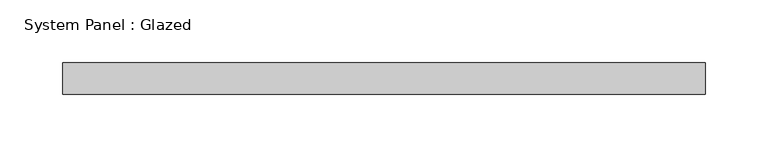
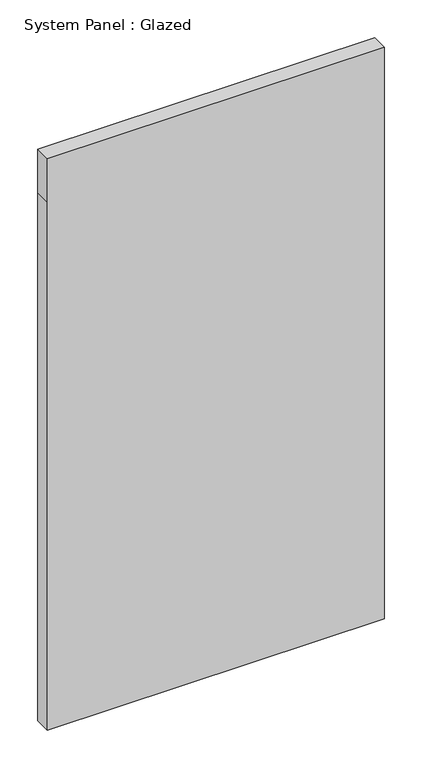
"""IFC4 building model written with IfcOpenShell, lengths in millimetres: plate geometry, System Panel : Glazed."""

from ifc_helpers import new_model, si_unit, frame, origin, place, context, project, spatial, polyline, outline, extrude, source, transform, mapped, element, save


def system_panel_glazed_706913d7(model_context):
    return source(origin(), model_context, "Body", "SweptSolid", [
        extrude(outline(polyline([(0.0, -257.175), (0.0, 257.175), (852.6761324, 257.175), (922.5261324, 257.175), (922.5261324, -257.175), (852.6761324, -257.175), (0.0, -257.175)])), frame((0.0, 19.05, 0.0), z_axis=(0.0, 1.0, 0.0), x_axis=(0.0, 0.0, 1.0)), (0.0, 0.0, 1.0), 25.4),
    ])


if __name__ == "__main__":
    model = new_model("IFC4")
    model_context = context("Model", 3, world=origin())
    ifc_project = project(units=[si_unit("LENGTHUNIT", "METRE", prefix="MILLI")], contexts=[model_context])
    site = spatial("IfcSite", under=ifc_project)
    building = spatial("IfcBuilding", under=site)
    placement = place(None, origin())
    system_panel_glazed_shape = system_panel_glazed_706913d7(model_context)
    element("IfcPlate", 1, ObjectType="System Panel : Glazed", at=placement, inside=building, context=model_context, shape_type="MappedRepresentation", body=[
        mapped(system_panel_glazed_shape, transform((0.0, 0.0, 0.0), x_axis=(1.0, 0.0, 0.0), y_axis=(0.0, 1.0, 0.0), z_axis=(0.0, 0.0, 1.0))),
    ])
    save(model, "model.ifc")

# Revit data of these elements
# Type "System Panel : Glazed"
#   Construction Type Id = "GSP4R"
#   Analytic Construction = "1/8 in Pilkington single glazing"
#   Visual Light Transmittance = 0.9
#   Solar Heat Gain Coefficient = 0.86
#   Heat Transfer Coefficient (U) = 1.18115 BTU/(h·ft²·°F)
#   Define Thermal Properties by = 1
# Element 1 (IfcPlate, "System Panel : Glazed")
#   Materials on its faces: "Glass"
# Materials
#   "Glass": class "Glass", colour RGB 0 128 192, transparency 0.75, Description = "Soda Lime Glass", Cost = 0
